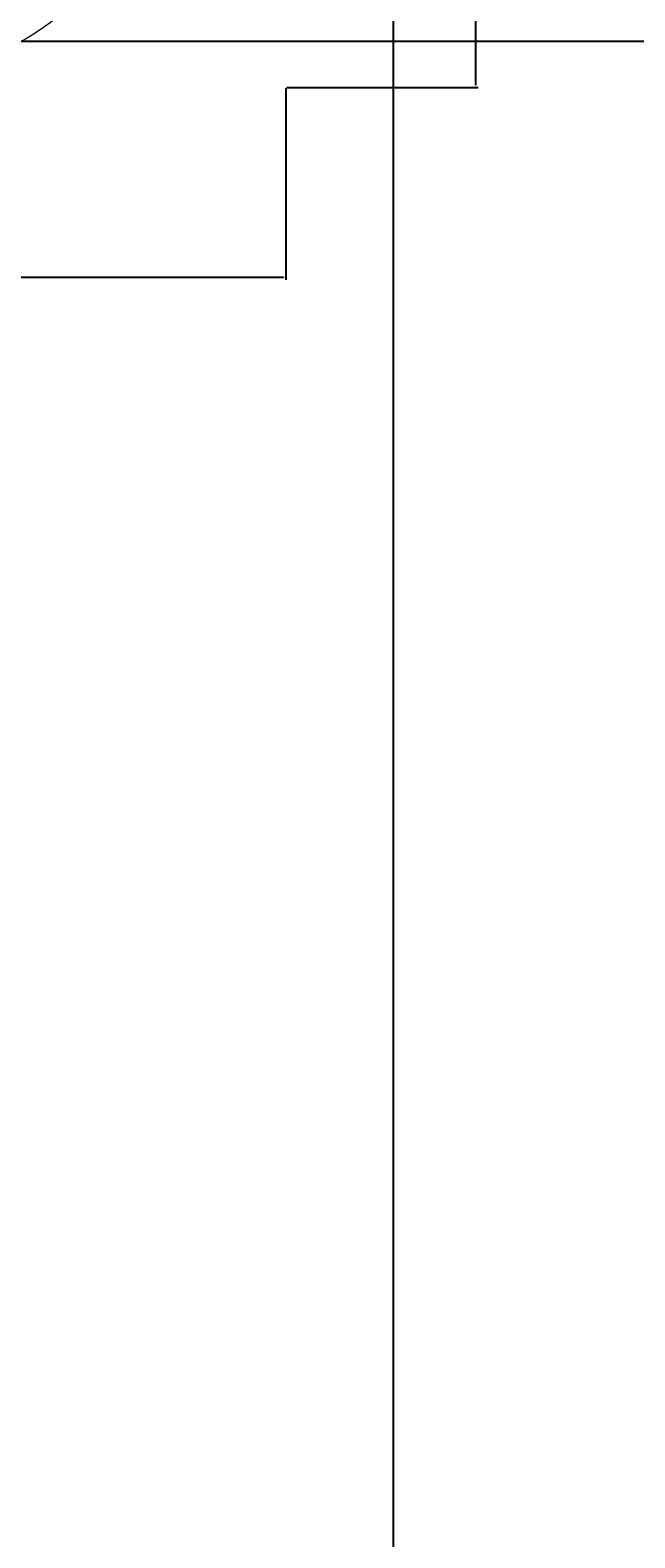
# Model space of a CAD drawing. Units: inches. Extents: x -61 to 1599, y -1316 to 257.
# Tile 93 of 204: x 321 to 367, y -280 to -166. Entities that reach past the tile are written whole.
import ezdxf

# ---------------------------------------------------------------- set-up
doc = ezdxf.new("R2010")
doc.units = ezdxf.units.IN
doc.header["$MEASUREMENT"] = 0
doc.layers.add('A-ANNO-DIMS', color=2, linetype='Continuous', lineweight=18)
doc.layers.add('FURNITURE', color=83, linetype='Continuous', lineweight=18)
doc.styles.get("Standard").update_dxf_attribs({"font": 'arial.ttf'})
doc.dimstyles.get("Standard").update_dxf_attribs({"dimtxt": 0.18, "dimasz": 0.18, "dimexe": 0.18, "dimexo": 0.0625, "dimgap": 0.09, "dimtad": 0, "dimtih": 1, "dimtoh": 1, "dimdec": 0, "dimzin": 0, "dimdsep": 46, "dimlunit": 3, "dimtxsty": 'Standard', "dimcen": 0.09, "dimadec": 0, "dimazin": 0, "dimtfac": 1, "dimtdec": 0, "dimtofl": 0, "dimtmove": 0, "dimatfit": 3, "dimfxl": 1, "dimtolj": 1, "dimtzin": 0, "dimarcsym": 0})

# ---------------------------------------------------------------- blocks, each defined once
blk = doc.blocks.new('DINING-TABLE-OVAL')
for p, q in [((20.06, 34.26), (38.12, 65.35)), ((20.69, 45.86), (30.12, 61.18)), ((27.51, 37.68), (36.94, 53.01))]:
    blk.add_line(p, q)
for centre, radius, start, end in [((28.99, 70.07), 25.36, 35.5172, 144.4828), ((85.79, 47.89), 85.79, 154.5151, 205.4849), ((-21.85, 47.89), 80.45, 332.689, 27.311), ((28.99, 24.89), 24.89, 213.9753, 326.0247)]:
    blk.add_arc(centre, radius, start, end)
blk = doc.blocks.new('*D666')
at = {"layer": 'A-ANNO-DIMS', "color": 0, "lineweight": -2, "transparency": 16777216}
for p, q in [((340.28, -75.2), (354.71, -75.2)), ((354.53, -75.38), (354.53, -122.73)), ((354.53, -170.45), (354.53, -123.09)), ((340.28, -170.63), (354.71, -170.63))]:
    blk.add_line(p, q, dxfattribs=at)
at = {"layer": 'A-ANNO-DIMS', "color": 0, "transparency": 16777216}
for points in [[(354.5, -75.38), (354.56, -75.38), (354.53, -75.2)], [(354.5, -170.45), (354.56, -170.45), (354.53, -170.63)]]:
    blk.add_solid(points, dxfattribs=at)
at = {"layer": 'DEFPOINTS', "color": 0, "transparency": 16777216}
for p in [(340.22, -75.2), (354.53, -75.2), (340.22, -170.63)]:
    blk.add_point(p, dxfattribs=at)
at = {"layer": 'A-ANNO-DIMS', "color": 0, "transparency": 16777216, "insert": (354.53, -122.91), "char_height": 0.18, "attachment_point": 5}
blk.add_mtext('\\A1;DINING TABLE 95 TYP.', dxfattribs=at)
blk = doc.blocks.new('*D667')
at = {"layer": 'A-ANNO-DIMS', "color": 0, "lineweight": -2, "transparency": 16777216}
for p, q in [((275.85, -170.69), (275.85, -185.12)), ((340.22, -170.69), (340.22, -185.12)), ((276.03, -184.94), (307.51, -184.94)), ((340.04, -184.94), (308.56, -184.94))]:
    blk.add_line(p, q, dxfattribs=at)
at = {"layer": 'A-ANNO-DIMS', "color": 0, "transparency": 16777216}
for points in [[(276.03, -184.91), (276.03, -184.97), (275.85, -184.94)], [(340.04, -184.91), (340.04, -184.97), (340.22, -184.94)]]:
    blk.add_solid(points, dxfattribs=at)
at = {"layer": 'DEFPOINTS', "color": 0, "transparency": 16777216}
for p in [(275.85, -170.63), (340.22, -170.63), (340.22, -184.94)]:
    blk.add_point(p, dxfattribs=at)
at = {"layer": 'A-ANNO-DIMS', "color": 0, "transparency": 16777216, "insert": (308.04, -184.94), "char_height": 0.18, "attachment_point": 5}
blk.add_mtext('\\A1;64 TYP.', dxfattribs=at)
blk = doc.blocks.new('*D699')
at = {"layer": 'A-ANNO-DIMS', "color": 0, "lineweight": -2, "transparency": 16777216}
for p, q in [((835.64, -167.17), (-61.08, -167.17)), ((-60.9, -167.35), (-60.9, -306.73)), ((-60.9, -446.47), (-60.9, -307.09)), ((841.64, -446.65), (-61.08, -446.65))]:
    blk.add_line(p, q, dxfattribs=at)
at = {"layer": 'A-ANNO-DIMS', "color": 0, "transparency": 16777216}
for points in [[(-60.93, -167.35), (-60.87, -167.35), (-60.9, -167.17)], [(-60.93, -446.47), (-60.87, -446.47), (-60.9, -446.65)]]:
    blk.add_solid(points, dxfattribs=at)
at = {"layer": 'DEFPOINTS', "color": 0, "transparency": 16777216}
for p in [(835.7, -167.17), (-60.9, -446.65), (841.7, -446.65)]:
    blk.add_point(p, dxfattribs=at)
at = {"layer": 'A-ANNO-DIMS', "color": 0, "transparency": 16777216, "insert": (-60.9, -306.91), "char_height": 0.18, "attachment_point": 5}
blk.add_mtext('\\A1;279.5', dxfattribs=at)
blk = doc.blocks.new('*D702')
at = {"layer": 'A-ANNO-DIMS', "color": 0, "lineweight": -2, "transparency": 16777216}
for p, q in [((276.88, -616.88), (276.88, 257.46)), ((277.06, 257.28), (312.21, 257.28)), ((348.14, 257.28), (312.99, 257.28)), ((348.32, -616.88), (348.32, 257.46))]:
    blk.add_line(p, q, dxfattribs=at)
at = {"layer": 'A-ANNO-DIMS', "color": 0, "transparency": 16777216}
for points in [[(277.06, 257.31), (277.06, 257.25), (276.88, 257.28)], [(348.14, 257.31), (348.14, 257.25), (348.32, 257.28)]]:
    blk.add_solid(points, dxfattribs=at)
at = {"layer": 'DEFPOINTS', "color": 0, "transparency": 16777216}
for p in [(348.32, 257.28), (276.88, -616.94), (348.32, -616.94)]:
    blk.add_point(p, dxfattribs=at)
at = {"layer": 'A-ANNO-DIMS', "color": 0, "transparency": 16777216, "insert": (312.6, 257.28), "char_height": 0.18, "attachment_point": 5}
blk.add_mtext('\\A1;71.44', dxfattribs=at)

msp = doc.modelspace()

# ---------------------------------------------------------------- block references
at = {"layer": 'FURNITURE'}
msp.add_blockref('DINING-TABLE-OVAL', (278.634, -170.626), dxfattribs=at)

# ---------------------------------------------------------------- dimensions: what is measured, and where the dimension line sits
at = {"layer": 'A-ANNO-DIMS'}
dim = msp.add_linear_dim(base=(348.3201, 257.2771), p1=(276.8825, -616.9446), p2=(348.3201, -616.9446), dimstyle='Standard', override={"dimdec": 2, "dimlfac": 1, "dimrnd": 0, "dimzin": 0, "dimdsep": 46, "dimlunit": 2}, dxfattribs=at)
dim.commit()
dim.dimension.update_dxf_attribs({"geometry": '*D702', "text_midpoint": (312.6013, 257.2771)})
dim = msp.add_linear_dim(base=(354.533, -75.1959), p1=(340.2185, -170.6256), p2=(340.2185, -75.1959), angle=90, text='DINING TABLE <> TYP.', dimstyle='Standard', override={"dimdec": 0, "dimlfac": 1, "dimrnd": 0, "dimzin": 0, "dimdsep": 46, "dimlunit": 2}, dxfattribs=at)
dim.commit()
dim.dimension.update_dxf_attribs({"geometry": '*D666', "text_midpoint": (354.533, -122.9108)})
dim = msp.add_linear_dim(base=(-60.8972, -446.6462), p1=(835.7028, -167.169), p2=(841.7028, -446.6462), angle=90, dimstyle='Standard', override={"dimdec": 1, "dimlfac": 1, "dimrnd": 0, "dimzin": 0, "dimdsep": 46, "dimlunit": 2}, dxfattribs=at)
dim.commit()
dim.dimension.update_dxf_attribs({"geometry": '*D699', "text_midpoint": (-60.8972, -306.9076)})
dim = msp.add_linear_dim(base=(340.2185, -184.9401), p1=(275.8519, -170.6256), p2=(340.2185, -170.6256), text='<> TYP.', dimstyle='Standard', override={"dimdec": 0, "dimlfac": 1, "dimrnd": 0, "dimzin": 0, "dimdsep": 46, "dimlunit": 2}, dxfattribs=at)
dim.commit()
dim.dimension.update_dxf_attribs({"geometry": '*D667', "text_midpoint": (308.0352, -184.9401)})

doc.saveas('drawing.dxf')
